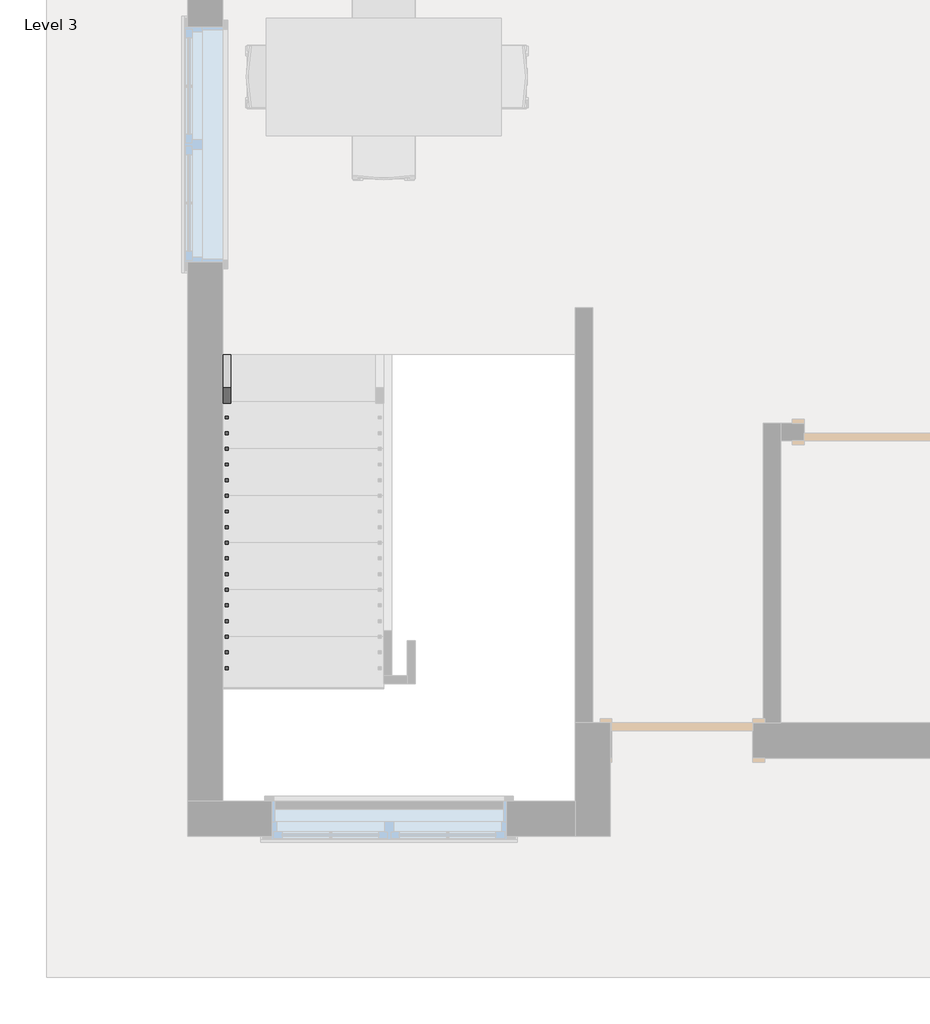
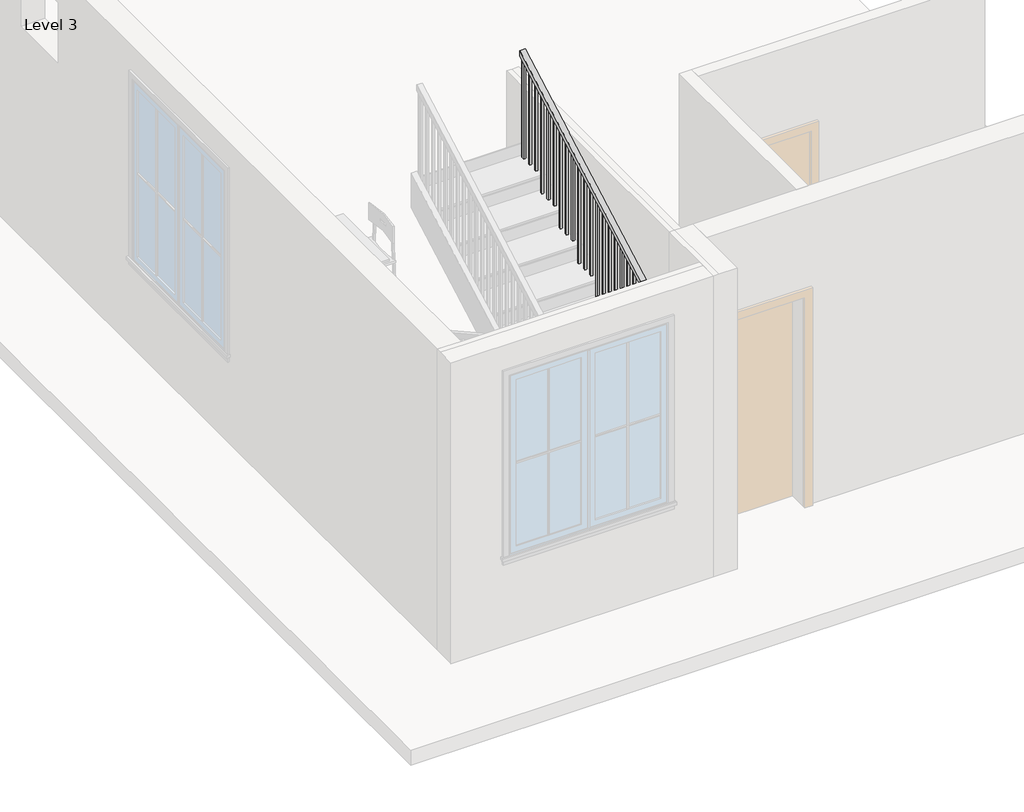
# One storey, part 2 of 3: 1 railing.
"""IFC4 building model written with IfcOpenShell, lengths in millimetres."""

from ifc_helpers import new_model, si_unit, frame, origin, place, context, project, spatial, polyline, outline, extrude, faceted_brep, element, save

model = new_model("IFC4")

# Units and contexts
model_context = context("Model", 3, world=origin())
ifc_project = project(units=[si_unit("LENGTHUNIT", "METRE", prefix="MILLI")], contexts=[model_context])

# Site, building, storey
site = spatial("IfcSite", under=ifc_project)
building = spatial("IfcBuilding", under=site)
storey = spatial("IfcBuildingStorey", under=building, Name="Level 3", Elevation=6248.4)

# Railing
placement = place(None, origin())
element("IfcRailing", 1, ObjectType="Handrail - Rectangular", at=placement, inside=storey, context=model_context, shape_type="SolidModel", body=[
    faceted_brep([(-4181.480864, -3571.6080018, 7332.1333333), (-4181.480864, -3571.6080018, 7274.020221), (-4232.280864, -3571.6080018, 7274.020221), (-4232.280864, -3571.6080018, 7332.1333333), (-4181.480864, -5705.2080018, 8517.4666667), (-4181.480864, -5718.371604, 8466.6666667), (-4232.280864, -5718.371604, 8466.6666667), (-4232.280864, -5705.2080018, 8517.4666667), (-4181.480864, -6416.4080018, 8517.4666667), (-4181.480864, -6416.4080018, 8466.6666667), (-4232.280864, -6467.2080018, 8466.6666667), (-4232.280864, -6467.2080018, 8517.4666667), (-1997.080864, -6416.4080018, 8517.4666667), (-1997.080864, -6416.4080018, 8466.6666667), (-1946.280864, -6467.2080018, 8466.6666667), (-1946.280864, -6467.2080018, 8517.4666667), (-1997.080864, -5705.2080018, 8517.4666667), (-1997.080864, -5692.0443995, 8466.6666667), (-1946.280864, -5692.0443995, 8466.6666667), (-1946.280864, -5705.2080018, 8517.4666667), (-1997.080864, -3571.6080018, 9702.8), (-1946.280864, -3571.6080018, 9702.8), (-1946.280864, -3571.6080018, 9644.6868876), (-1997.080864, -3571.6080018, 9644.6868876)], [[[0, 1, 2, 3]], [[1, 0, 4, 5]], [[2, 1, 5, 6]], [[3, 2, 6, 7]], [[0, 3, 7, 4]], [[5, 4, 8, 9]], [[6, 5, 9, 10]], [[7, 6, 10, 11]], [[4, 7, 11, 8]], [[9, 8, 12, 13]], [[10, 9, 13, 14]], [[11, 10, 14, 15]], [[8, 11, 15, 12]], [[13, 12, 16, 17]], [[14, 13, 17, 18]], [[15, 14, 18, 19]], [[12, 15, 19, 16]], [[20, 21, 22, 23]], [[17, 16, 20, 23]], [[18, 17, 23, 22]], [[19, 18, 22, 21]], [[16, 19, 21, 20]]]),
    extrude(outline(polyline([(-3606.5330018, 9625.2841099), (-3587.4830018, 9635.8674432), (-3587.4830018, 8619.0666667), (-3606.5330018, 8619.0666667), (-3606.5330018, 9625.2841099)])), frame((-1981.205864, 0.0, 0.0), z_axis=(1.0, 0.0, 0.0), x_axis=(0.0, 1.0, 0.0)), (0.0, 0.0, 1.0), 19.05),
    extrude(outline(polyline([(-3708.1330018, 9568.8396654), (-3689.0830018, 9579.4229988), (-3689.0830018, 8619.0666667), (-3708.1330018, 8619.0666667), (-3708.1330018, 9568.8396654)])), frame((-1981.205864, 0.0, 0.0), z_axis=(1.0, 0.0, 0.0), x_axis=(0.0, 1.0, 0.0)), (0.0, 0.0, 1.0), 19.05),
    extrude(outline(polyline([(-3809.7330018, 9512.395221), (-3790.6830018, 9522.9785543), (-3790.6830018, 8619.0666667), (-3809.7330018, 8619.0666667), (-3809.7330018, 9512.395221)])), frame((-1981.205864, 0.0, 0.0), z_axis=(1.0, 0.0, 0.0), x_axis=(0.0, 1.0, 0.0)), (0.0, 0.0, 1.0), 19.05),
    extrude(outline(polyline([(-3911.3330018, 9455.9507765), (-3892.2830018, 9466.5341099), (-3892.2830018, 8449.7333333), (-3911.3330018, 8449.7333333), (-3911.3330018, 9455.9507765)])), frame((-1981.205864, 0.0, 0.0), z_axis=(1.0, 0.0, 0.0), x_axis=(0.0, 1.0, 0.0)), (0.0, 0.0, 1.0), 19.05),
    extrude(outline(polyline([(-4012.9330018, 9399.5063321), (-3993.8830018, 9410.0896654), (-3993.8830018, 8449.7333333), (-4012.9330018, 8449.7333333), (-4012.9330018, 9399.5063321)])), frame((-1981.205864, 0.0, 0.0), z_axis=(1.0, 0.0, 0.0), x_axis=(0.0, 1.0, 0.0)), (0.0, 0.0, 1.0), 19.05),
    extrude(outline(polyline([(-4114.5330018, 9343.0618876), (-4095.4830018, 9353.645221), (-4095.4830018, 8449.7333333), (-4114.5330018, 8449.7333333), (-4114.5330018, 9343.0618876)])), frame((-1981.205864, 0.0, 0.0), z_axis=(1.0, 0.0, 0.0), x_axis=(0.0, 1.0, 0.0)), (0.0, 0.0, 1.0), 19.05),
    extrude(outline(polyline([(-4216.1330018, 9286.6174432), (-4197.0830018, 9297.2007765), (-4197.0830018, 8280.4), (-4216.1330018, 8280.4), (-4216.1330018, 9286.6174432)])), frame((-1981.205864, 0.0, 0.0), z_axis=(1.0, 0.0, 0.0), x_axis=(0.0, 1.0, 0.0)), (0.0, 0.0, 1.0), 19.05),
    extrude(outline(polyline([(-4317.7330018, 9230.1729988), (-4298.6830018, 9240.7563321), (-4298.6830018, 8280.4), (-4317.7330018, 8280.4), (-4317.7330018, 9230.1729988)])), frame((-1981.205864, 0.0, 0.0), z_axis=(1.0, 0.0, 0.0), x_axis=(0.0, 1.0, 0.0)), (0.0, 0.0, 1.0), 19.05),
    extrude(outline(polyline([(-4419.3330018, 9173.7285543), (-4400.2830018, 9184.3118876), (-4400.2830018, 8280.4), (-4419.3330018, 8280.4), (-4419.3330018, 9173.7285543)])), frame((-1981.205864, 0.0, 0.0), z_axis=(1.0, 0.0, 0.0), x_axis=(0.0, 1.0, 0.0)), (0.0, 0.0, 1.0), 19.05),
    extrude(outline(polyline([(-4520.9330018, 9117.2841099), (-4501.8830018, 9127.8674432), (-4501.8830018, 8111.0666667), (-4520.9330018, 8111.0666667), (-4520.9330018, 9117.2841099)])), frame((-1981.205864, 0.0, 0.0), z_axis=(1.0, 0.0, 0.0), x_axis=(0.0, 1.0, 0.0)), (0.0, 0.0, 1.0), 19.05),
    extrude(outline(polyline([(-4622.5330018, 9060.8396654), (-4603.4830018, 9071.4229988), (-4603.4830018, 8111.0666667), (-4622.5330018, 8111.0666667), (-4622.5330018, 9060.8396654)])), frame((-1981.205864, 0.0, 0.0), z_axis=(1.0, 0.0, 0.0), x_axis=(0.0, 1.0, 0.0)), (0.0, 0.0, 1.0), 19.05),
    extrude(outline(polyline([(-4724.1330018, 9004.395221), (-4705.0830018, 9014.9785543), (-4705.0830018, 8111.0666667), (-4724.1330018, 8111.0666667), (-4724.1330018, 9004.395221)])), frame((-1981.205864, 0.0, 0.0), z_axis=(1.0, 0.0, 0.0), x_axis=(0.0, 1.0, 0.0)), (0.0, 0.0, 1.0), 19.05),
    extrude(outline(polyline([(-4825.7330018, 8947.9507765), (-4806.6830018, 8958.5341099), (-4806.6830018, 7941.7333333), (-4825.7330018, 7941.7333333), (-4825.7330018, 8947.9507765)])), frame((-1981.205864, 0.0, 0.0), z_axis=(1.0, 0.0, 0.0), x_axis=(0.0, 1.0, 0.0)), (0.0, 0.0, 1.0), 19.05),
    extrude(outline(polyline([(-4927.3330018, 8891.5063321), (-4908.2830018, 8902.0896654), (-4908.2830018, 7941.7333333), (-4927.3330018, 7941.7333333), (-4927.3330018, 8891.5063321)])), frame((-1981.205864, 0.0, 0.0), z_axis=(1.0, 0.0, 0.0), x_axis=(0.0, 1.0, 0.0)), (0.0, 0.0, 1.0), 19.05),
    extrude(outline(polyline([(-5028.9330018, 8835.0618876), (-5009.8830018, 8845.645221), (-5009.8830018, 7941.7333333), (-5028.9330018, 7941.7333333), (-5028.9330018, 8835.0618876)])), frame((-1981.205864, 0.0, 0.0), z_axis=(1.0, 0.0, 0.0), x_axis=(0.0, 1.0, 0.0)), (0.0, 0.0, 1.0), 19.05),
    extrude(outline(polyline([(-5130.5330018, 8778.6174432), (-5111.4830018, 8789.2007765), (-5111.4830018, 7772.4), (-5130.5330018, 7772.4), (-5130.5330018, 8778.6174432)])), frame((-1981.205864, 0.0, 0.0), z_axis=(1.0, 0.0, 0.0), x_axis=(0.0, 1.0, 0.0)), (0.0, 0.0, 1.0), 19.05),
    extrude(outline(polyline([(-5232.1330018, 8722.1729988), (-5213.0830018, 8732.7563321), (-5213.0830018, 7772.4), (-5232.1330018, 7772.4), (-5232.1330018, 8722.1729988)])), frame((-1981.205864, 0.0, 0.0), z_axis=(1.0, 0.0, 0.0), x_axis=(0.0, 1.0, 0.0)), (0.0, 0.0, 1.0), 19.05),
    extrude(outline(polyline([(-5333.7330018, 8665.7285543), (-5314.6830018, 8676.3118876), (-5314.6830018, 7772.4), (-5333.7330018, 7772.4), (-5333.7330018, 8665.7285543)])), frame((-1981.205864, 0.0, 0.0), z_axis=(1.0, 0.0, 0.0), x_axis=(0.0, 1.0, 0.0)), (0.0, 0.0, 1.0), 19.05),
    extrude(outline(polyline([(-5435.3330018, 8609.2841099), (-5416.2830018, 8619.8674432), (-5416.2830018, 7603.0666667), (-5435.3330018, 7603.0666667), (-5435.3330018, 8609.2841099)])), frame((-1981.205864, 0.0, 0.0), z_axis=(1.0, 0.0, 0.0), x_axis=(0.0, 1.0, 0.0)), (0.0, 0.0, 1.0), 19.05),
    extrude(outline(polyline([(-5536.9330018, 8552.8396654), (-5517.8830018, 8563.4229988), (-5517.8830018, 7603.0666667), (-5536.9330018, 7603.0666667), (-5536.9330018, 8552.8396654)])), frame((-1981.205864, 0.0, 0.0), z_axis=(1.0, 0.0, 0.0), x_axis=(0.0, 1.0, 0.0)), (0.0, 0.0, 1.0), 19.05),
    extrude(outline(polyline([(-5638.5330018, 8496.395221), (-5619.4830018, 8506.9785543), (-5619.4830018, 7603.0666667), (-5638.5330018, 7603.0666667), (-5638.5330018, 8496.395221)])), frame((-1981.205864, 0.0, 0.0), z_axis=(1.0, 0.0, 0.0), x_axis=(0.0, 1.0, 0.0)), (0.0, 0.0, 1.0), 19.05),
    extrude(outline(polyline([(-1962.155864, -5740.1330018), (-1981.205864, -5740.1330018), (-1981.205864, -5721.0830018), (-1962.155864, -5721.0830018), (-1962.155864, -5740.1330018)])), frame((0.0, 0.0, 7603.0666667), z_axis=(0.0, 0.0, 1.0), x_axis=(1.0, 0.0, 0.0)), (0.0, 0.0, 1.0), 863.6),
    extrude(outline(polyline([(-1962.155864, -5841.7330018), (-1981.205864, -5841.7330018), (-1981.205864, -5822.6830018), (-1962.155864, -5822.6830018), (-1962.155864, -5841.7330018)])), frame((0.0, 0.0, 7603.0666667), z_axis=(0.0, 0.0, 1.0), x_axis=(1.0, 0.0, 0.0)), (0.0, 0.0, 1.0), 863.6),
    extrude(outline(polyline([(-1962.155864, -5943.3330018), (-1981.205864, -5943.3330018), (-1981.205864, -5924.2830018), (-1962.155864, -5924.2830018), (-1962.155864, -5943.3330018)])), frame((0.0, 0.0, 7603.0666667), z_axis=(0.0, 0.0, 1.0), x_axis=(1.0, 0.0, 0.0)), (0.0, 0.0, 1.0), 863.6),
    extrude(outline(polyline([(-1962.155864, -6044.9330018), (-1981.205864, -6044.9330018), (-1981.205864, -6025.8830018), (-1962.155864, -6025.8830018), (-1962.155864, -6044.9330018)])), frame((0.0, 0.0, 7603.0666667), z_axis=(0.0, 0.0, 1.0), x_axis=(1.0, 0.0, 0.0)), (0.0, 0.0, 1.0), 863.6),
    extrude(outline(polyline([(-1962.155864, -6146.5330018), (-1981.205864, -6146.5330018), (-1981.205864, -6127.4830018), (-1962.155864, -6127.4830018), (-1962.155864, -6146.5330018)])), frame((0.0, 0.0, 7603.0666667), z_axis=(0.0, 0.0, 1.0), x_axis=(1.0, 0.0, 0.0)), (0.0, 0.0, 1.0), 863.6),
    extrude(outline(polyline([(-1962.155864, -6248.1330018), (-1981.205864, -6248.1330018), (-1981.205864, -6229.0830018), (-1962.155864, -6229.0830018), (-1962.155864, -6248.1330018)])), frame((0.0, 0.0, 7603.0666667), z_axis=(0.0, 0.0, 1.0), x_axis=(1.0, 0.0, 0.0)), (0.0, 0.0, 1.0), 863.6),
    extrude(outline(polyline([(-1962.155864, -6349.7330018), (-1981.205864, -6349.7330018), (-1981.205864, -6330.6830018), (-1962.155864, -6330.6830018), (-1962.155864, -6349.7330018)])), frame((0.0, 0.0, 7603.0666667), z_axis=(0.0, 0.0, 1.0), x_axis=(1.0, 0.0, 0.0)), (0.0, 0.0, 1.0), 863.6),
    extrude(outline(polyline([(-2082.805864, -6451.3330018), (-2082.805864, -6432.2830018), (-2063.755864, -6432.2830018), (-2063.755864, -6451.3330018), (-2082.805864, -6451.3330018)])), frame((0.0, 0.0, 7603.0666667), z_axis=(0.0, 0.0, 1.0), x_axis=(1.0, 0.0, 0.0)), (0.0, 0.0, 1.0), 863.6),
    extrude(outline(polyline([(-2184.405864, -6451.3330018), (-2184.405864, -6432.2830018), (-2165.355864, -6432.2830018), (-2165.355864, -6451.3330018), (-2184.405864, -6451.3330018)])), frame((0.0, 0.0, 7603.0666667), z_axis=(0.0, 0.0, 1.0), x_axis=(1.0, 0.0, 0.0)), (0.0, 0.0, 1.0), 863.6),
    extrude(outline(polyline([(-2286.005864, -6451.3330018), (-2286.005864, -6432.2830018), (-2266.955864, -6432.2830018), (-2266.955864, -6451.3330018), (-2286.005864, -6451.3330018)])), frame((0.0, 0.0, 7603.0666667), z_axis=(0.0, 0.0, 1.0), x_axis=(1.0, 0.0, 0.0)), (0.0, 0.0, 1.0), 863.6),
    extrude(outline(polyline([(-2387.605864, -6451.3330018), (-2387.605864, -6432.2830018), (-2368.555864, -6432.2830018), (-2368.555864, -6451.3330018), (-2387.605864, -6451.3330018)])), frame((0.0, 0.0, 7603.0666667), z_axis=(0.0, 0.0, 1.0), x_axis=(1.0, 0.0, 0.0)), (0.0, 0.0, 1.0), 863.6),
    extrude(outline(polyline([(-2489.205864, -6451.3330018), (-2489.205864, -6432.2830018), (-2470.155864, -6432.2830018), (-2470.155864, -6451.3330018), (-2489.205864, -6451.3330018)])), frame((0.0, 0.0, 7603.0666667), z_axis=(0.0, 0.0, 1.0), x_axis=(1.0, 0.0, 0.0)), (0.0, 0.0, 1.0), 863.6),
    extrude(outline(polyline([(-2590.805864, -6451.3330018), (-2590.805864, -6432.2830018), (-2571.755864, -6432.2830018), (-2571.755864, -6451.3330018), (-2590.805864, -6451.3330018)])), frame((0.0, 0.0, 7603.0666667), z_axis=(0.0, 0.0, 1.0), x_axis=(1.0, 0.0, 0.0)), (0.0, 0.0, 1.0), 863.6),
    extrude(outline(polyline([(-2692.405864, -6451.3330018), (-2692.405864, -6432.2830018), (-2673.355864, -6432.2830018), (-2673.355864, -6451.3330018), (-2692.405864, -6451.3330018)])), frame((0.0, 0.0, 7603.0666667), z_axis=(0.0, 0.0, 1.0), x_axis=(1.0, 0.0, 0.0)), (0.0, 0.0, 1.0), 863.6),
    extrude(outline(polyline([(-2794.005864, -6451.3330018), (-2794.005864, -6432.2830018), (-2774.955864, -6432.2830018), (-2774.955864, -6451.3330018), (-2794.005864, -6451.3330018)])), frame((0.0, 0.0, 7603.0666667), z_axis=(0.0, 0.0, 1.0), x_axis=(1.0, 0.0, 0.0)), (0.0, 0.0, 1.0), 863.6),
    extrude(outline(polyline([(-2895.605864, -6451.3330018), (-2895.605864, -6432.2830018), (-2876.555864, -6432.2830018), (-2876.555864, -6451.3330018), (-2895.605864, -6451.3330018)])), frame((0.0, 0.0, 7603.0666667), z_axis=(0.0, 0.0, 1.0), x_axis=(1.0, 0.0, 0.0)), (0.0, 0.0, 1.0), 863.6),
    extrude(outline(polyline([(-2997.205864, -6451.3330018), (-2997.205864, -6432.2830018), (-2978.155864, -6432.2830018), (-2978.155864, -6451.3330018), (-2997.205864, -6451.3330018)])), frame((0.0, 0.0, 7603.0666667), z_axis=(0.0, 0.0, 1.0), x_axis=(1.0, 0.0, 0.0)), (0.0, 0.0, 1.0), 863.6),
    extrude(outline(polyline([(-3098.805864, -6451.3330018), (-3098.805864, -6432.2830018), (-3079.755864, -6432.2830018), (-3079.755864, -6451.3330018), (-3098.805864, -6451.3330018)])), frame((0.0, 0.0, 7603.0666667), z_axis=(0.0, 0.0, 1.0), x_axis=(1.0, 0.0, 0.0)), (0.0, 0.0, 1.0), 863.6),
    extrude(outline(polyline([(-3200.405864, -6451.3330018), (-3200.405864, -6432.2830018), (-3181.355864, -6432.2830018), (-3181.355864, -6451.3330018), (-3200.405864, -6451.3330018)])), frame((0.0, 0.0, 7603.0666667), z_axis=(0.0, 0.0, 1.0), x_axis=(1.0, 0.0, 0.0)), (0.0, 0.0, 1.0), 863.6),
    extrude(outline(polyline([(-3302.005864, -6451.3330018), (-3302.005864, -6432.2830018), (-3282.955864, -6432.2830018), (-3282.955864, -6451.3330018), (-3302.005864, -6451.3330018)])), frame((0.0, 0.0, 7603.0666667), z_axis=(0.0, 0.0, 1.0), x_axis=(1.0, 0.0, 0.0)), (0.0, 0.0, 1.0), 863.6),
    extrude(outline(polyline([(-3403.605864, -6451.3330018), (-3403.605864, -6432.2830018), (-3384.555864, -6432.2830018), (-3384.555864, -6451.3330018), (-3403.605864, -6451.3330018)])), frame((0.0, 0.0, 7603.0666667), z_axis=(0.0, 0.0, 1.0), x_axis=(1.0, 0.0, 0.0)), (0.0, 0.0, 1.0), 863.6),
    extrude(outline(polyline([(-3505.205864, -6451.3330018), (-3505.205864, -6432.2830018), (-3486.155864, -6432.2830018), (-3486.155864, -6451.3330018), (-3505.205864, -6451.3330018)])), frame((0.0, 0.0, 7603.0666667), z_axis=(0.0, 0.0, 1.0), x_axis=(1.0, 0.0, 0.0)), (0.0, 0.0, 1.0), 863.6),
    extrude(outline(polyline([(-3606.805864, -6451.3330018), (-3606.805864, -6432.2830018), (-3587.755864, -6432.2830018), (-3587.755864, -6451.3330018), (-3606.805864, -6451.3330018)])), frame((0.0, 0.0, 7603.0666667), z_axis=(0.0, 0.0, 1.0), x_axis=(1.0, 0.0, 0.0)), (0.0, 0.0, 1.0), 863.6),
    extrude(outline(polyline([(-3708.405864, -6451.3330018), (-3708.405864, -6432.2830018), (-3689.355864, -6432.2830018), (-3689.355864, -6451.3330018), (-3708.405864, -6451.3330018)])), frame((0.0, 0.0, 7603.0666667), z_axis=(0.0, 0.0, 1.0), x_axis=(1.0, 0.0, 0.0)), (0.0, 0.0, 1.0), 863.6),
    extrude(outline(polyline([(-3810.005864, -6451.3330018), (-3810.005864, -6432.2830018), (-3790.955864, -6432.2830018), (-3790.955864, -6451.3330018), (-3810.005864, -6451.3330018)])), frame((0.0, 0.0, 7603.0666667), z_axis=(0.0, 0.0, 1.0), x_axis=(1.0, 0.0, 0.0)), (0.0, 0.0, 1.0), 863.6),
    extrude(outline(polyline([(-3911.605864, -6451.3330018), (-3911.605864, -6432.2830018), (-3892.555864, -6432.2830018), (-3892.555864, -6451.3330018), (-3911.605864, -6451.3330018)])), frame((0.0, 0.0, 7603.0666667), z_axis=(0.0, 0.0, 1.0), x_axis=(1.0, 0.0, 0.0)), (0.0, 0.0, 1.0), 863.6),
    extrude(outline(polyline([(-4013.205864, -6451.3330018), (-4013.205864, -6432.2830018), (-3994.155864, -6432.2830018), (-3994.155864, -6451.3330018), (-4013.205864, -6451.3330018)])), frame((0.0, 0.0, 7603.0666667), z_axis=(0.0, 0.0, 1.0), x_axis=(1.0, 0.0, 0.0)), (0.0, 0.0, 1.0), 863.6),
    extrude(outline(polyline([(-4114.805864, -6451.3330018), (-4114.805864, -6432.2830018), (-4095.755864, -6432.2830018), (-4095.755864, -6451.3330018), (-4114.805864, -6451.3330018)])), frame((0.0, 0.0, 7603.0666667), z_axis=(0.0, 0.0, 1.0), x_axis=(1.0, 0.0, 0.0)), (0.0, 0.0, 1.0), 863.6),
    extrude(outline(polyline([(-4216.405864, -6406.8830018), (-4197.355864, -6406.8830018), (-4197.355864, -6425.9330018), (-4216.405864, -6425.9330018), (-4216.405864, -6406.8830018)])), frame((0.0, 0.0, 7603.0666667), z_axis=(0.0, 0.0, 1.0), x_axis=(1.0, 0.0, 0.0)), (0.0, 0.0, 1.0), 863.6),
    extrude(outline(polyline([(-4216.405864, -6305.2830018), (-4197.355864, -6305.2830018), (-4197.355864, -6324.3330018), (-4216.405864, -6324.3330018), (-4216.405864, -6305.2830018)])), frame((0.0, 0.0, 7603.0666667), z_axis=(0.0, 0.0, 1.0), x_axis=(1.0, 0.0, 0.0)), (0.0, 0.0, 1.0), 863.6),
    extrude(outline(polyline([(-4216.405864, -6203.6830018), (-4197.355864, -6203.6830018), (-4197.355864, -6222.7330018), (-4216.405864, -6222.7330018), (-4216.405864, -6203.6830018)])), frame((0.0, 0.0, 7603.0666667), z_axis=(0.0, 0.0, 1.0), x_axis=(1.0, 0.0, 0.0)), (0.0, 0.0, 1.0), 863.6),
    extrude(outline(polyline([(-4216.405864, -6102.0830018), (-4197.355864, -6102.0830018), (-4197.355864, -6121.1330018), (-4216.405864, -6121.1330018), (-4216.405864, -6102.0830018)])), frame((0.0, 0.0, 7603.0666667), z_axis=(0.0, 0.0, 1.0), x_axis=(1.0, 0.0, 0.0)), (0.0, 0.0, 1.0), 863.6),
    extrude(outline(polyline([(-4216.405864, -6000.4830018), (-4197.355864, -6000.4830018), (-4197.355864, -6019.5330018), (-4216.405864, -6019.5330018), (-4216.405864, -6000.4830018)])), frame((0.0, 0.0, 7603.0666667), z_axis=(0.0, 0.0, 1.0), x_axis=(1.0, 0.0, 0.0)), (0.0, 0.0, 1.0), 863.6),
    extrude(outline(polyline([(-4216.405864, -5898.8830018), (-4197.355864, -5898.8830018), (-4197.355864, -5917.9330018), (-4216.405864, -5917.9330018), (-4216.405864, -5898.8830018)])), frame((0.0, 0.0, 7603.0666667), z_axis=(0.0, 0.0, 1.0), x_axis=(1.0, 0.0, 0.0)), (0.0, 0.0, 1.0), 863.6),
    extrude(outline(polyline([(-4216.405864, -5797.2830018), (-4197.355864, -5797.2830018), (-4197.355864, -5816.3330018), (-4216.405864, -5816.3330018), (-4216.405864, -5797.2830018)])), frame((0.0, 0.0, 7603.0666667), z_axis=(0.0, 0.0, 1.0), x_axis=(1.0, 0.0, 0.0)), (0.0, 0.0, 1.0), 863.6),
    extrude(outline(polyline([(-5714.7330018, 8464.645221), (-5695.6830018, 8454.0618876), (-5695.6830018, 7603.0666667), (-5714.7330018, 7603.0666667), (-5714.7330018, 8464.645221)])), frame((-4216.405864, 0.0, 0.0), z_axis=(1.0, 0.0, 0.0), x_axis=(0.0, 1.0, 0.0)), (0.0, 0.0, 1.0), 19.05),
    extrude(outline(polyline([(-5613.1330018, 8408.2007765), (-5594.0830018, 8397.6174432), (-5594.0830018, 7433.7333333), (-5613.1330018, 7433.7333333), (-5613.1330018, 8408.2007765)])), frame((-4216.405864, 0.0, 0.0), z_axis=(1.0, 0.0, 0.0), x_axis=(0.0, 1.0, 0.0)), (0.0, 0.0, 1.0), 19.05),
    extrude(outline(polyline([(-5511.5330018, 8351.7563321), (-5492.4830018, 8341.1729988), (-5492.4830018, 7433.7333333), (-5511.5330018, 7433.7333333), (-5511.5330018, 8351.7563321)])), frame((-4216.405864, 0.0, 0.0), z_axis=(1.0, 0.0, 0.0), x_axis=(0.0, 1.0, 0.0)), (0.0, 0.0, 1.0), 19.05),
    extrude(outline(polyline([(-5409.9330018, 8295.3118876), (-5390.8830018, 8284.7285543), (-5390.8830018, 7433.7333333), (-5409.9330018, 7433.7333333), (-5409.9330018, 8295.3118876)])), frame((-4216.405864, 0.0, 0.0), z_axis=(1.0, 0.0, 0.0), x_axis=(0.0, 1.0, 0.0)), (0.0, 0.0, 1.0), 19.05),
    extrude(outline(polyline([(-5308.3330018, 8238.8674432), (-5289.2830018, 8228.2841099), (-5289.2830018, 7264.4), (-5308.3330018, 7264.4), (-5308.3330018, 8238.8674432)])), frame((-4216.405864, 0.0, 0.0), z_axis=(1.0, 0.0, 0.0), x_axis=(0.0, 1.0, 0.0)), (0.0, 0.0, 1.0), 19.05),
    extrude(outline(polyline([(-5206.7330018, 8182.4229988), (-5187.6830018, 8171.8396654), (-5187.6830018, 7264.4), (-5206.7330018, 7264.4), (-5206.7330018, 8182.4229988)])), frame((-4216.405864, 0.0, 0.0), z_axis=(1.0, 0.0, 0.0), x_axis=(0.0, 1.0, 0.0)), (0.0, 0.0, 1.0), 19.05),
    extrude(outline(polyline([(-5105.1330018, 8125.9785543), (-5086.0830018, 8115.395221), (-5086.0830018, 7264.4), (-5105.1330018, 7264.4), (-5105.1330018, 8125.9785543)])), frame((-4216.405864, 0.0, 0.0), z_axis=(1.0, 0.0, 0.0), x_axis=(0.0, 1.0, 0.0)), (0.0, 0.0, 1.0), 19.05),
    extrude(outline(polyline([(-5003.5330018, 8069.5341099), (-4984.4830018, 8058.9507765), (-4984.4830018, 7095.0666667), (-5003.5330018, 7095.0666667), (-5003.5330018, 8069.5341099)])), frame((-4216.405864, 0.0, 0.0), z_axis=(1.0, 0.0, 0.0), x_axis=(0.0, 1.0, 0.0)), (0.0, 0.0, 1.0), 19.05),
    extrude(outline(polyline([(-4901.9330018, 8013.0896654), (-4882.8830018, 8002.5063321), (-4882.8830018, 7095.0666667), (-4901.9330018, 7095.0666667), (-4901.9330018, 8013.0896654)])), frame((-4216.405864, 0.0, 0.0), z_axis=(1.0, 0.0, 0.0), x_axis=(0.0, 1.0, 0.0)), (0.0, 0.0, 1.0), 19.05),
    extrude(outline(polyline([(-4800.3330018, 7956.645221), (-4781.2830018, 7946.0618876), (-4781.2830018, 7095.0666667), (-4800.3330018, 7095.0666667), (-4800.3330018, 7956.645221)])), frame((-4216.405864, 0.0, 0.0), z_axis=(1.0, 0.0, 0.0), x_axis=(0.0, 1.0, 0.0)), (0.0, 0.0, 1.0), 19.05),
    extrude(outline(polyline([(-4698.7330018, 7900.2007765), (-4679.6830018, 7889.6174432), (-4679.6830018, 6925.7333333), (-4698.7330018, 6925.7333333), (-4698.7330018, 7900.2007765)])), frame((-4216.405864, 0.0, 0.0), z_axis=(1.0, 0.0, 0.0), x_axis=(0.0, 1.0, 0.0)), (0.0, 0.0, 1.0), 19.05),
    extrude(outline(polyline([(-4597.1330018, 7843.7563321), (-4578.0830018, 7833.1729988), (-4578.0830018, 6925.7333333), (-4597.1330018, 6925.7333333), (-4597.1330018, 7843.7563321)])), frame((-4216.405864, 0.0, 0.0), z_axis=(1.0, 0.0, 0.0), x_axis=(0.0, 1.0, 0.0)), (0.0, 0.0, 1.0), 19.05),
    extrude(outline(polyline([(-4495.5330018, 7787.3118876), (-4476.4830018, 7776.7285543), (-4476.4830018, 6925.7333333), (-4495.5330018, 6925.7333333), (-4495.5330018, 7787.3118876)])), frame((-4216.405864, 0.0, 0.0), z_axis=(1.0, 0.0, 0.0), x_axis=(0.0, 1.0, 0.0)), (0.0, 0.0, 1.0), 19.05),
    extrude(outline(polyline([(-4393.9330018, 7730.8674432), (-4374.8830018, 7720.2841099), (-4374.8830018, 6756.4), (-4393.9330018, 6756.4), (-4393.9330018, 7730.8674432)])), frame((-4216.405864, 0.0, 0.0), z_axis=(1.0, 0.0, 0.0), x_axis=(0.0, 1.0, 0.0)), (0.0, 0.0, 1.0), 19.05),
    extrude(outline(polyline([(-4292.3330018, 7674.4229988), (-4273.2830018, 7663.8396654), (-4273.2830018, 6756.4), (-4292.3330018, 6756.4), (-4292.3330018, 7674.4229988)])), frame((-4216.405864, 0.0, 0.0), z_axis=(1.0, 0.0, 0.0), x_axis=(0.0, 1.0, 0.0)), (0.0, 0.0, 1.0), 19.05),
    extrude(outline(polyline([(-4190.7330018, 7617.9785543), (-4171.6830018, 7607.395221), (-4171.6830018, 6756.4), (-4190.7330018, 6756.4), (-4190.7330018, 7617.9785543)])), frame((-4216.405864, 0.0, 0.0), z_axis=(1.0, 0.0, 0.0), x_axis=(0.0, 1.0, 0.0)), (0.0, 0.0, 1.0), 19.05),
    extrude(outline(polyline([(-4089.1330018, 7561.5341099), (-4070.0830018, 7550.9507765), (-4070.0830018, 6587.0666667), (-4089.1330018, 6587.0666667), (-4089.1330018, 7561.5341099)])), frame((-4216.405864, 0.0, 0.0), z_axis=(1.0, 0.0, 0.0), x_axis=(0.0, 1.0, 0.0)), (0.0, 0.0, 1.0), 19.05),
    extrude(outline(polyline([(-3987.5330018, 7505.0896654), (-3968.4830018, 7494.5063321), (-3968.4830018, 6587.0666667), (-3987.5330018, 6587.0666667), (-3987.5330018, 7505.0896654)])), frame((-4216.405864, 0.0, 0.0), z_axis=(1.0, 0.0, 0.0), x_axis=(0.0, 1.0, 0.0)), (0.0, 0.0, 1.0), 19.05),
    extrude(outline(polyline([(-3885.9330018, 7448.645221), (-3866.8830018, 7438.0618876), (-3866.8830018, 6587.0666667), (-3885.9330018, 6587.0666667), (-3885.9330018, 7448.645221)])), frame((-4216.405864, 0.0, 0.0), z_axis=(1.0, 0.0, 0.0), x_axis=(0.0, 1.0, 0.0)), (0.0, 0.0, 1.0), 19.05),
    extrude(outline(polyline([(-3784.3330018, 7392.2007765), (-3765.2830018, 7381.6174432), (-3765.2830018, 6417.7333333), (-3784.3330018, 6417.7333333), (-3784.3330018, 7392.2007765)])), frame((-4216.405864, 0.0, 0.0), z_axis=(1.0, 0.0, 0.0), x_axis=(0.0, 1.0, 0.0)), (0.0, 0.0, 1.0), 19.05),
    extrude(outline(polyline([(-3682.7330018, 7335.7563321), (-3663.6830018, 7325.1729988), (-3663.6830018, 6417.7333333), (-3682.7330018, 6417.7333333), (-3682.7330018, 7335.7563321)])), frame((-4216.405864, 0.0, 0.0), z_axis=(1.0, 0.0, 0.0), x_axis=(0.0, 1.0, 0.0)), (0.0, 0.0, 1.0), 19.05),
    extrude(outline(polyline([(-1981.205864, -6451.3330018), (-1981.205864, -6432.2830018), (-1962.155864, -6432.2830018), (-1962.155864, -6451.3330018), (-1981.205864, -6451.3330018)])), frame((0.0, 0.0, 7603.0666667), z_axis=(0.0, 0.0, 1.0), x_axis=(1.0, 0.0, 0.0)), (0.0, 0.0, 1.0), 863.6),
    extrude(outline(polyline([(-4216.405864, -6432.2830018), (-4197.355864, -6432.2830018), (-4197.355864, -6451.3330018), (-4216.405864, -6451.3330018), (-4216.405864, -6432.2830018)])), frame((0.0, 0.0, 7603.0666667), z_axis=(0.0, 0.0, 1.0), x_axis=(1.0, 0.0, 0.0)), (0.0, 0.0, 1.0), 863.6),
    extrude(outline(polyline([(-3590.6580018, 9634.1035543), (-3571.6080018, 9644.6868876), (-3571.6080018, 8619.0666667), (-3590.6580018, 8619.0666667), (-3590.6580018, 9634.1035543)])), frame((-1981.205864, 0.0, 0.0), z_axis=(1.0, 0.0, 0.0), x_axis=(0.0, 1.0, 0.0)), (0.0, 0.0, 1.0), 19.05),
    extrude(outline(polyline([(-3590.6580018, 7284.6035543), (-3571.6080018, 7274.020221), (-3571.6080018, 6417.7333333), (-3590.6580018, 6417.7333333), (-3590.6580018, 7284.6035543)])), frame((-4216.405864, 0.0, 0.0), z_axis=(1.0, 0.0, 0.0), x_axis=(0.0, 1.0, 0.0)), (0.0, 0.0, 1.0), 19.05),
])

save(model, "model.ifc")

# Revit data of these elements
# Type "Handrail - Rectangular"
#   Assembly Code = "C2010400"
#   built-in parameter 1008612 = 0.0416667 (stored number, unit not read)
#   built-in parameter 1008611 = 0.0416667 (stored number, unit not read)
#   built-in parameter 1008609 = 0.333333 (stored number, unit not read)
#   built-in parameter 1008604 = 0.166667 (stored number, unit not read)
#   built-in parameter 1008603 = 0.166667 (stored number, unit not read)
#   Railing Height = 3' - 0"
#   built-in parameter 1008630 = 2
#   built-in parameter 1008610 = 2
#   built-in parameter 1008618 = Baluster - Square : 3/4"
# Element 1 (IfcRailing, "Handrail - Rectangular")
#   Phase Created = New Construction
